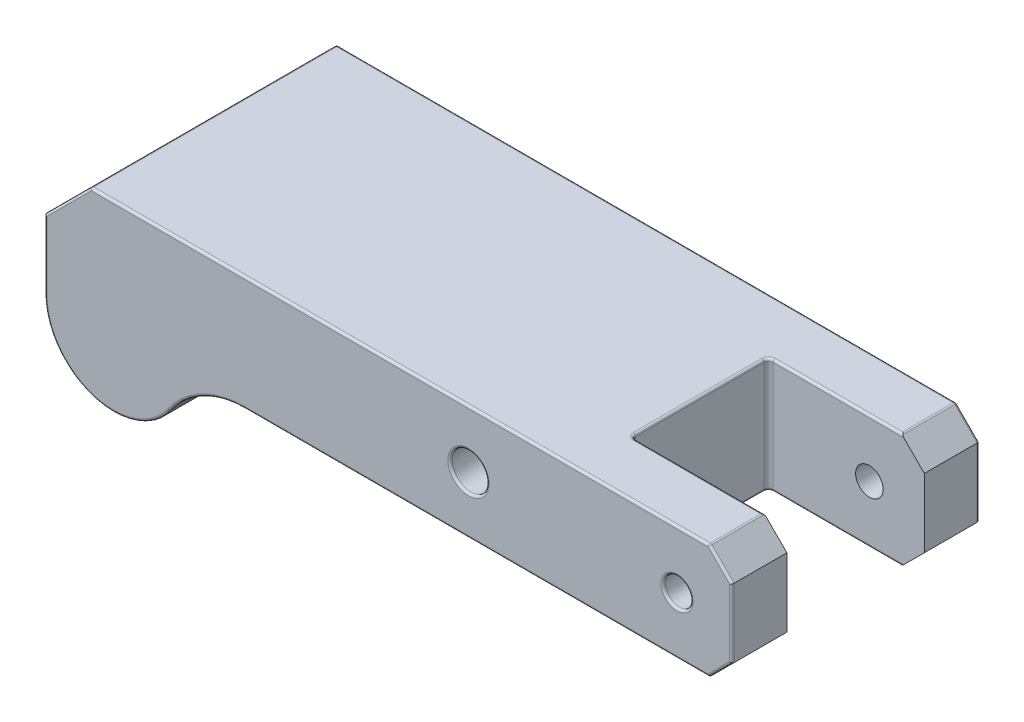
from build123d import *

# Parameters (mm, degrees)
ARM_BODY_54MM_DEPTH      = 27
FORK_SLOT_SKETCH_W       = 34
FORK_SLOT_SKETCH_H       = 30
FORK_SLOT_12MM_DEPTH     = 54
END_CHAMFER_5MM_SIZE     = 5
CORNER_CHAMFER_10MM_SIZE = 10
PIN_HOLES_SKETCH_R       = 4
PIN_HOLES_SKETCH_R_2     = 3
PIN_HOLES_DEPTH          = 54
SLOT_FILLET_R1_R         = 1
EDGE_FILLET_R0_5_A_R     = 0.5
EDGE_FILLET_R0_5_B_R     = 0.5


with BuildPart() as part:
    # Arm Profile Sketch → Arm Body 54mm (new, symmetric)
    with BuildSketch(Plane.XY):
        with BuildLine():
            Line((0, 0), (-48.107006044, 0))
            ThreePointArc((-48.107006044, 0), (-57.365207042, -2.271894791), (-64.520042177, -8.571428571))
            ThreePointArc((-64.520042177, -8.571428571), (-81.321664305, -14.311650088), (-91.829819277, 0))
            Line((-91.829819277, 0), (-91.829819277, 25))
            Line((-91.829819277, 25), (58.170180723, 25))
            Line((58.170180723, 25), (58.170180723, 0))
            Line((58.170180723, 0), (0, 0))
        make_face()
    extrude(amount=ARM_BODY_54MM_DEPTH, both=True)

    # Fork Slot Sketch → Fork Slot 12mm (cut)
    with BuildSketch(Plane(origin=(0, 25, 0), x_dir=(1, 0, 0), z_dir=(0, 1, 0))):
        with Locations((41.170180723, 0)):
            Rectangle(FORK_SLOT_SKETCH_W, FORK_SLOT_SKETCH_H)
    extrude(amount=-FORK_SLOT_12MM_DEPTH, mode=Mode.SUBTRACT)

    # End Chamfer 5mm
    end_chamfer_5mm_edges = [part.edges().sort_by_distance(p)[0] for p in [
        (58.170180723, 25, 21),
        (58.170180723, 0, 21),
        (58.170180723, 0, -21),
        (58.170180723, 25, -21),
    ]]
    chamfer(end_chamfer_5mm_edges, length=END_CHAMFER_5MM_SIZE)

    # Corner Chamfer 10mm
    corner_chamfer_10mm_edges = [part.edges().sort_by_distance(p)[0] for p in [
        (-91.829819277, 25, 0),
    ]]
    chamfer(corner_chamfer_10mm_edges, length=CORNER_CHAMFER_10MM_SIZE)

    # Pin Holes Sketch → Pin Holes (cut)
    with BuildSketch(Plane.XY.offset(27)):
        with Locations((0.670180723, 12.5)):
            Circle(PIN_HOLES_SKETCH_R)
        with Locations((46.170180723, 12.5)):
            Circle(PIN_HOLES_SKETCH_R_2)
    extrude(amount=-PIN_HOLES_DEPTH, mode=Mode.SUBTRACT)

    # Slot Fillet R1
    slot_fillet_r1_edges = [part.edges().sort_by_distance(p)[0] for p in [
        (24.170180723, 12.5, 15),
        (24.170180723, 12.5, -15),
    ]]
    fillet(slot_fillet_r1_edges, radius=SLOT_FILLET_R1_R)

    # Edge Fillet R0.5 A
    edge_fillet_r0_5_a_edges = [part.edges().sort_by_distance(p)[0] for p in [
        (-81.321664305, -14.311650088, 27),
        (-57.365207042, -2.271894791, 27),
        (58.170180723, 12.5, -27),
        (-14.329819277, 25, -27),
        (55.670180723, 22.5, -27),
        (55.670180723, 2.5, -27),
        (2.531587339, 0, 27),
        (58.170180723, 12.5, 27),
        (-14.329819277, 25, 27),
        (55.670180723, 22.5, 27),
        (55.670180723, 2.5, 27),
        (-91.829819277, 7.5, -27),
        (-91.829819277, 7.5, 27),
        (-86.829819277, 20, -27),
        (-86.829819277, 20, 27),
        (2.531587339, 0, -27),
        (-57.365207042, -2.271894791, -27),
        (-3.329819277, 12.5, -27),
        (-3.329819277, 12.5, 27),
        (43.170180723, 12.5, -27),
        (43.170180723, 12.5, 27),
        (-81.321664305, -14.311650088, -27),
    ]]
    fillet(edge_fillet_r0_5_a_edges, radius=EDGE_FILLET_R0_5_A_R)

    # Edge Fillet R0.5 B
    edge_fillet_r0_5_b_edges = [part.edges().sort_by_distance(p)[0] for p in [
        (53.170180723, 25, 20.75),
        (53.170180723, 0, -20.75),
        (-81.829819277, 25, 0),
        (53.106600299, 0.153496722, 26.860465641),
        (-81.766238853, 24.846503278, 26.860465641),
        (53.106600299, 24.846503278, 26.860465641),
        (53.106600299, 24.846503278, -26.860465641),
        (-81.766238853, 24.846503278, -26.860465641),
        (53.106600299, 0.153496722, -26.860465641),
        (39.170180723, 0, -15),
        (53.170180723, 0, 20.75),
        (39.170180723, 25, -15),
        (53.170180723, 25, -20.75),
        (24.170180723, 25, 0),
        (24.170180723, 0, 0),
        (39.170180723, 0, 15),
        (39.170180723, 25, 15),
        (24.463073942, 25, -14.707106781),
        (24.463073942, 0, -14.707106781),
        (24.463073942, 25, 14.707106781),
        (24.463073942, 0, 14.707106781),
    ]]
    fillet(edge_fillet_r0_5_b_edges, radius=EDGE_FILLET_R0_5_B_R)


solid = part.part
